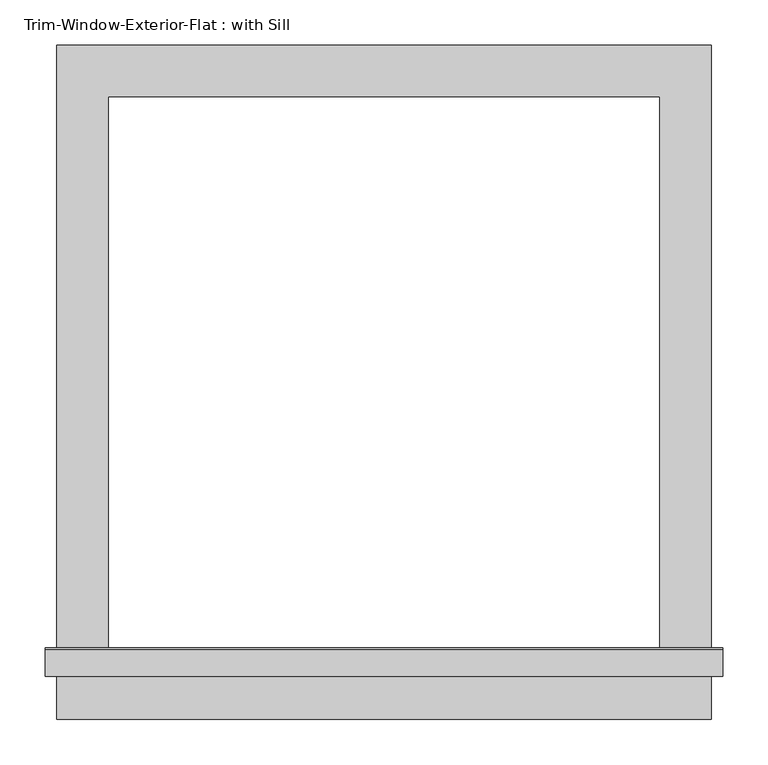
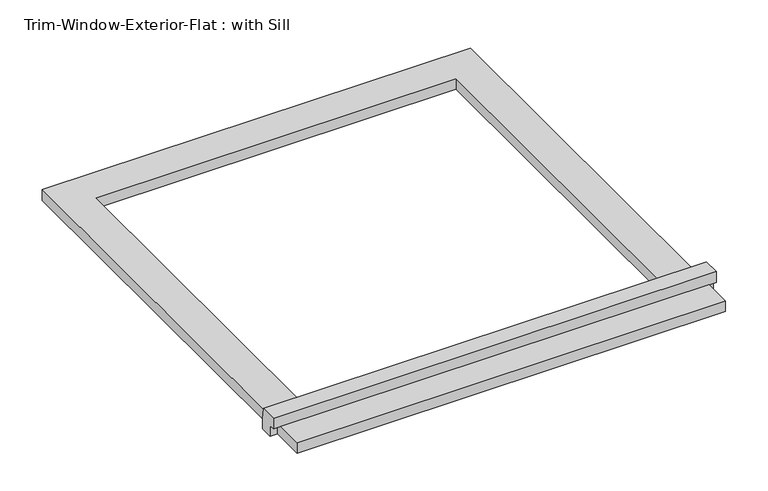
"""IFC4 building model written with IfcOpenShell, lengths in millimetres: proxy geometry, Trim-Window-Exterior-Flat : with Sill."""

from ifc_helpers import new_model, si_unit, frame, origin, origin_with_axes, place, context, project, spatial, polyline, outline, extrude, source, transform, mapped, element, save


def trim_window_exterior_flat_with_sill_858dc10d(model_context):
    return source(origin(), model_context, "Body", "SweptSolid", [
        extrude(outline(polyline([(361.95, -631.7823709), (361.95, -688.9323709), (-361.95, -688.9323709), (-361.95, -631.7823709), (361.95, -631.7823709)])), origin_with_axes(), (0.0, 0.0, 1.0), 19.05),
        extrude(outline(polyline([(-641.35, 38.1), (-612.0580645, 38.1), (-609.6, 19.05), (-609.6, 0.0), (-631.7823709, 0.0), (-631.7823709, 19.05), (-641.35, 19.05), (-641.35, 38.1)])), frame((-374.65, 0.0, 0.0), z_axis=(1.0, 0.0, 0.0), x_axis=(0.0, 1.0, 0.0)), (0.0, 0.0, 1.0), 749.3),
        extrude(outline(polyline([(-361.95, 57.15), (361.95, 57.15), (361.95, -609.6), (304.8, -609.6), (304.8, 0.0), (-304.8, 0.0), (-304.8, -609.6), (-361.95, -609.6), (-361.95, 57.15)])), origin_with_axes(), (0.0, 0.0, 1.0), 19.05),
    ])


if __name__ == "__main__":
    model = new_model("IFC4")
    model_context = context("Model", 3, world=origin())
    ifc_project = project(units=[si_unit("LENGTHUNIT", "METRE", prefix="MILLI")], contexts=[model_context])
    site = spatial("IfcSite", under=ifc_project)
    building = spatial("IfcBuilding", under=site)
    placement = place(None, origin())
    trim_window_exterior_flat_with_sill_shape = trim_window_exterior_flat_with_sill_858dc10d(model_context)
    element("IfcBuildingElementProxy", 1, Name="Trim-Window-Exterior-Flat : with Sill", ObjectType="Trim-Window-Exterior-Flat : with Sill", at=placement, inside=building, context=model_context, shape_type="MappedRepresentation", body=[
        mapped(trim_window_exterior_flat_with_sill_shape, transform((0.0, 0.0, 0.0), x_axis=(1.0, 0.0, 0.0), y_axis=(0.0, 1.0, 0.0), z_axis=(0.0, 0.0, 1.0))),
    ])
    save(model, "model.ifc")

# Revit data of these elements
# Type "Trim-Window-Exterior-Flat : with Sill"
#   Trim Width = 0' - 2 1/4"
#   Trim Thickness_Picture Frame = 0' - 1 1/4"
#   Trim Thickness_with Sill = 0' - 0 3/4"
#   Sill Thickness = 0' - 1 1/4"
#   Opening Width [instance default] = 2' - 0"
#   Opening Height [instance default] = 3' - 0"
#   Default Elevation = 4' - 0"
#   Sill = yes
#   Picture Frame = no
#   Trim Material [instance default] = none
# Element 1 (IfcBuildingElementProxy, "Trim-Window-Exterior-Flat : with Sill")
#   Opening Height = 2' - 0"
#   Trim Material = Clad - White
#   Materials on its faces: "Clad - White"
# Materials
#   "Clad - White": class "Wood", colour RGB 242 242 238, transparency 0, Cost = 0
